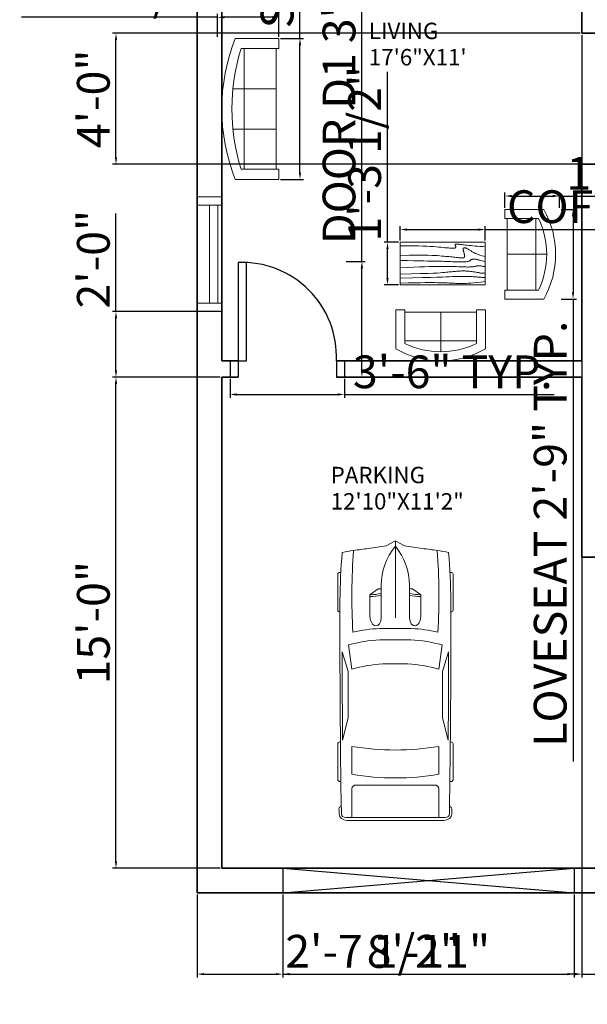
# Model space of a CAD drawing. Units: inches. Extents: x 2011 to 2548, y 530 to 1188.
# Tile 1 of 5: x 2011 to 2220, y 530 to 891. Entities that reach past the tile are written whole.
import ezdxf

# ---------------------------------------------------------------- set-up
doc = ezdxf.new("R2010")
doc.units = ezdxf.units.IN
for name, color, linetype, lineweight in [('A-ANNO-DIMS', 2, 'Continuous', 18), ('A-AREA-IDEN', 7, 'Continuous', 25), ('A-DOOR', 3, 'Continuous', 25), ('A-FURN', 8, 'Continuous', 18), ('A-GLAZ', 4, 'Continuous', 18), ('A-SITE-VEHC', 8, 'Continuous', 13), ('A-WALL', 7, 'Continuous', 35)]:
    doc.layers.add(name, color=color, linetype=linetype, lineweight=lineweight)
doc.styles.get("Standard").update_dxf_attribs({"font": 'arial.ttf'})
doc.dimstyles.new('ISO-25', dxfattribs={"dimtxt": 12, "dimasz": 2.5, "dimexe": 1.25, "dimexo": 0.625, "dimtad": 1, "dimdec": 1, "dimlunit": 3, "dimtxsty": 'Standard', "dimcen": 2.5, "dimadec": 0, "dimazin": 0, "dimtfac": 1, "dimtdec": 1, "dimtmove": 0, "dimatfit": 3, "dimfxl": 1, "dimarcsym": 0})

# ---------------------------------------------------------------- blocks, each defined once
blk = doc.blocks.new('Sofa - Roundback 7 ft.')
for p, q in [((-36.000027, -34), (-36.000027, -11.4696)), ((-12.00002, -32.4421), (-12.00003, -6.5971)), ((11.99997, -32.4421), (11.99998, -6.5971)), ((35.99998, -34), (35.99998, -11.4696)), ((-35.999844, -13.3819), (35.9998, -13.3819)), ((-36.000027, -32.4421), (35.99998, -32.4421))]:
    blk.add_line(p, q)
for points in [[(-36.000027, -34), (-42.000027, -34), (-42.000027, -8)], [(41.99998, -8), (41.99998, -34), (35.99998, -34)]]:
    blk.add_lwpolyline(points)
for centre, radius, start, end in [((0, -114.25), 114.25, 68.43141, 111.5686), ((-0.00001, -127.1968), 121.1968, 72.72033, 107.2797)]:
    blk.add_arc(centre, radius, start, end)
blk = doc.blocks.new('Table - Rectangular Woodgrain 60 x 30 in.')
for p, q in [((0, 0), (0, -30)), ((60, 0), (0, 0)), ((60, -30), (60, 0)), ((0, -30), (60, -30))]:
    blk.add_line(p, q)
for points in [[(0, -2.4), (4.8155, -2.418), (9.0302, -2.4688), (12.709, -2.5477), (15.9167, -2.65), (18.7181, -2.7711), (21.1781, -2.9063), (23.3616, -3.0508), (25.3333, -3.2), (27.1477, -3.3495), (28.8172, -3.4958), (30.3437, -3.636), (31.7291, -3.7667), (32.9756, -3.8849), (34.0849, -3.9875), (35.059, -4.0714), (35.9, -4.1334), (36.6114, -4.1711), (37.2041, -4.1854), (37.6906, -4.1779), (38.0833, -4.15), (38.3948, -4.1034), (38.6375, -4.0396), (38.8239, -3.9602), (38.9666, -3.8667), (39.0764, -3.7608), (39.1573, -3.6448), (39.2116, -3.521), (39.2416, -3.3917), (39.2498, -3.2593), (39.2385, -3.1261), (39.21, -2.9944), (39.1666, -2.8667), (39.111, -2.7447), (39.0468, -2.6281), (38.978, -2.5163), (38.9083, -2.4083), (38.8418, -2.3035), (38.7823, -2.201), (38.7337, -2.1001), (38.7, -2), (38.6844, -1.9003), (38.6875, -1.8021), (38.7094, -1.707), (38.75, -1.6167), (38.8094, -1.5326), (38.8875, -1.4563), (38.9844, -1.3893), (39.1, -1.3333), (39.2351, -1.2896), (39.3937, -1.2583), (39.5804, -1.2396), (39.8, -1.2333), (40.057, -1.2396), (40.3562, -1.2583), (40.7023, -1.2896), (41.1, -1.3333), (41.5547, -1.3895), (42.0755, -1.4573), (42.6721, -1.5361), (43.3542, -1.625), (44.1316, -1.7233), (45.014, -1.8302), (46.0114, -1.9449), (47.1333, -2.0667), (48.3862, -2.1947), (49.7625, -2.3281), (51.2513, -2.4663), (52.8416, -2.6083), (54.5226, -2.7535), (56.2833, -2.9011), (58.1127, -3.0501), (60, -3.2)], [(0, -9.2), (6.5759, -9.0858), (11.9385, -9.0365), (16.2527, -9.0418), (19.6833, -9.0917), (22.3952, -9.1759), (24.5531, -9.2844), (26.322, -9.4069), (27.8666, -9.5333), (29.3241, -9.6553), (30.7203, -9.7719), (32.0532, -9.8837), (33.3208, -9.9917), (34.5213, -10.0965), (35.6526, -10.199), (36.7128, -10.2999), (37.7, -10.4), (38.6129, -10.4996), (39.4531, -10.5969), (40.223, -10.6895), (40.925, -10.775), (41.5613, -10.8512), (42.1344, -10.9156), (42.6465, -10.966), (43.1, -11), (43.4976, -11.0158), (43.8437, -11.0136), (44.143, -10.9942), (44.4, -10.9583), (44.6195, -10.9069), (44.8062, -10.8406), (44.9648, -10.7603), (45.1, -10.6667), (45.2155, -10.5598), (45.3114, -10.4365), (45.3871, -10.2929), (45.4416, -10.125), (45.4743, -9.929), (45.4844, -9.7011), (45.4709, -9.4371), (45.4333, -9.1333), (45.3716, -8.7883), (45.2896, -8.4104), (45.1919, -8.0107), (45.0833, -7.6), (44.9685, -7.1893), (44.8521, -6.7896), (44.7388, -6.4117), (44.6333, -6.0667), (44.54, -5.7628), (44.4614, -5.4979), (44.4001, -5.2675), (44.3583, -5.0667), (44.3384, -4.8909), (44.3427, -4.7354), (44.3736, -4.5956), (44.4333, -4.4667), (44.5236, -4.3453), (44.6427, -4.2333), (44.7884, -4.1339), (44.9583, -4.05), (45.1501, -3.9849), (45.3614, -3.9417), (45.59, -3.9234), (45.8333, -3.9333), (46.0915, -3.9749), (46.3734, -4.0531), (46.6906, -4.1736), (47.0542, -4.3417), (47.4756, -4.5629), (47.9661, -4.8427), (48.5372, -5.1866), (49.2, -5.6), (49.9676, -6.0844), (50.8594, -6.625), (51.8965, -7.2031), (53.1, -7.8), (54.491, -8.3969), (56.0906, -8.975), (57.9199, -9.5156), (60, -10)], [(0, -12.8), (5.1847, -12.9322), (9.6213, -13.0323), (13.3963, -13.1059), (16.5958, -13.1583), (19.3063, -13.1952), (21.614, -13.2219), (23.6054, -13.2439), (25.3666, -13.2667), (26.9728, -13.2947), (28.4531, -13.3281), (29.8256, -13.3663), (31.1083, -13.4083), (32.3191, -13.4535), (33.476, -13.501), (34.597, -13.5501), (35.7, -13.6), (36.7984, -13.6497), (37.8875, -13.6979), (38.9578, -13.743), (40, -13.7833), (41.0047, -13.8174), (41.9625, -13.8438), (42.864, -13.8607), (43.7, -13.8667), (44.4631, -13.8604), (45.1552, -13.8417), (45.7801, -13.8104), (46.3416, -13.7667), (46.8439, -13.7104), (47.2906, -13.6417), (47.6858, -13.5604), (48.0333, -13.4667), (48.3375, -13.3608), (48.6042, -13.2448), (48.8396, -13.121), (49.05, -12.9917), (49.2417, -12.8593), (49.4208, -12.7261), (49.5937, -12.5944), (49.7667, -12.4667), (49.9452, -12.3451), (50.1323, -12.2313), (50.3303, -12.1268), (50.5416, -12.0333), (50.7686, -11.9524), (51.0135, -11.8854), (51.2788, -11.8341), (51.5666, -11.8), (51.8785, -11.7843), (52.2116, -11.7865), (52.562, -11.8059), (52.926, -11.8417), (53.2998, -11.8931), (53.6795, -11.9594), (54.0614, -12.0397), (54.4416, -12.1333), (54.8223, -12.2401), (55.2293, -12.3625), (55.6942, -12.5037), (56.2489, -12.6667), (56.9251, -12.8547), (57.7545, -13.0708), (58.7689, -13.3182), (60, -13.6)], [(0, -18), (5.124, -17.7273), (9.6609, -17.5057), (13.6705, -17.3303), (17.2125, -17.1958), (20.3467, -17.0973), (23.1328, -17.0297), (25.6307, -16.9878), (27.9, -16.9667), (29.9928, -16.9617), (31.9302, -16.9703), (33.7254, -16.9907), (35.3917, -17.0208), (36.9423, -17.0588), (38.3906, -17.1026), (39.7499, -17.1503), (41.0333, -17.2), (42.2519, -17.2496), (43.4073, -17.2969), (44.4986, -17.3395), (45.525, -17.375), (46.4858, -17.4012), (47.3802, -17.4156), (48.2074, -17.416), (48.9667, -17.4), (49.6583, -17.3662), (50.2872, -17.3167), (50.8595, -17.2547), (51.3812, -17.1833), (51.8584, -17.1057), (52.2971, -17.025), (52.7034, -16.9443), (53.0833, -16.8667), (53.443, -16.7951), (53.789, -16.7313), (54.128, -16.6768), (54.4666, -16.6334), (54.8115, -16.6024), (55.1693, -16.5854), (55.5465, -16.5841), (55.95, -16.6), (56.3828, -16.6337), (56.8346, -16.6823), (57.2915, -16.7418), (57.7396, -16.8084), (58.165, -16.878), (58.5539, -16.9469), (58.8924, -17.0111), (59.1666, -17.0667), (59.3679, -17.1107), (59.5078, -17.1438), (59.6032, -17.1675), (59.6708, -17.1833), (59.7275, -17.193), (59.7901, -17.1979), (59.8753, -17.1998), (60, -17.2)], [(0, -22.4), (8.0098, -22.2501), (14.4094, -22.1011), (19.4168, -21.9535), (23.25, -21.8083), (26.1269, -21.6663), (28.2656, -21.5281), (29.884, -21.3947), (31.2, -21.2667), (32.3967, -21.1448), (33.5172, -21.0292), (34.5697, -20.9198), (35.5625, -20.8167), (36.5037, -20.7198), (37.4015, -20.6292), (38.2642, -20.5448), (39.1, -20.4667), (39.9164, -20.3951), (40.7187, -20.3313), (41.5117, -20.2768), (42.3, -20.2333), (43.0883, -20.2024), (43.8812, -20.1854), (44.6836, -20.1841), (45.5, -20.2), (46.3328, -20.234), (47.1747, -20.2844), (48.0163, -20.3488), (48.8479, -20.425), (49.66, -20.5106), (50.4429, -20.6031), (51.1872, -20.7004), (51.8833, -20.8), (52.5246, -20.8999), (53.1166, -20.9995), (53.6681, -21.0983), (54.1875, -21.1958), (54.6834, -21.2919), (55.1646, -21.3859), (55.6394, -21.4777), (56.1167, -21.5667), (56.6028, -21.6515), (57.0961, -21.7266), (57.5929, -21.7852), (58.0896, -21.8208), (58.5823, -21.8268), (59.0674, -21.7964), (59.5412, -21.723), (60, -21.6)], [(0, -25.2), (8.6355, -25.0504), (15.7026, -24.9031), (21.4049, -24.7606), (25.9458, -24.625), (29.529, -24.4988), (32.3578, -24.3844), (34.6359, -24.284), (36.5667, -24.2), (38.3213, -24.1341), (39.9417, -24.0854), (41.437, -24.0523), (42.8167, -24.0333), (44.0901, -24.0268), (45.2667, -24.0313), (46.3557, -24.0451), (47.3667, -24.0667), (48.309, -24.0947), (49.1928, -24.1287), (50.0284, -24.168), (50.826, -24.2125), (51.5959, -24.2617), (52.3483, -24.3151), (53.0935, -24.3725), (53.8417, -24.4334), (54.6009, -24.497), (55.3699, -24.561), (56.1454, -24.6226), (56.9239, -24.6792), (57.7021, -24.7279), (58.4764, -24.7662), (59.2435, -24.7911), (60, -24.8)], [(0, -28.8), (5.6867, -28.6681), (10.45, -28.5698), (14.407, -28.5012), (17.675, -28.4584), (20.3711, -28.4374), (22.6125, -28.4344), (24.5164, -28.4455), (26.2, -28.4667), (27.762, -28.4947), (29.2276, -28.5281), (30.6033, -28.5663), (31.8958, -28.6084), (33.1118, -28.6535), (34.2578, -28.7011), (35.3405, -28.7501), (36.3666, -28.8), (37.3443, -28.8497), (38.288, -28.8974), (39.2137, -28.9412), (40.1375, -28.9792), (41.0753, -29.0093), (42.0432, -29.0297), (43.0572, -29.0384), (44.1333, -29.0333), (45.2936, -29.0114), (46.5843, -28.9641), (48.0579, -28.8816), (49.7666, -28.7542), (51.7629, -28.5721), (54.0989, -28.3255), (56.8272, -28.0048), (60, -27.6)]]:
    blk.add_lwpolyline(points)
blk = doc.blocks.new('Sofa - Roundback Loveseat 5 ft.')
for p, q in [((0, -32.44198), (0, -5.99998)), ((-24, -33.99998), (-24, -11.46958)), ((24.00004, -33.99998), (24.00004, -11.46958)), ((-23.9998, -13.38178), (23.99986, -13.38178)), ((-24, -32.44198), (24.00004, -32.44198))]:
    blk.add_line(p, q)
for points in [[(-24, -33.99998), (-30, -33.99998), (-30, -7.99998)], [(30.00004, -7.99998), (30.00004, -33.99998), (24.00004, -33.99998)]]:
    blk.add_lwpolyline(points)
for centre, radius, start, end in [((0, -60.24998), 60.24998, 60.13715, 119.8628), ((0, -61.38438), 55.38444, 64.32083, 115.6792)]:
    blk.add_arc(centre, radius, start, end)
blk = doc.blocks.new('*U11')
for p, q in [((21.1, 37.41), (21.1, 36.83)), ((46.55, 38.89), (22.35, 38.89)), ((47.8, 37.39), (47.8, 37.41)), ((87.99, 31.87), (74.76, 35.92)), ((134.31, 35.6), (119.29, 31.78)), ((135.45, 37.07), (135.45, 37.41)), ((136.7, 38.89), (160.9, 38.89)), ((162.15, 37.41), (162.15, 36.77)), ((186.47, -33.5), (186.47, 33.5)), ((70.03, 31.54), (86.41, 29.35)), ((138.42, 29.35), (157.25, 29.35)), ((186.47, 29.35), (167.01, 29.35)), ((188.4, -32.76), (188.4, 32.76)), ((164.52, 26.39), (164.52, -26.39)), ((32.27, 11.63), (36.13, 17.17)), ((36.13, 17.17), (50.94, 17.17)), ((29.77, 9.51), (51.68, 9.51)), ((32.12, 9.51), (32.12, 11.15)), ((58.92, -10.77), (58.92, 10.77)), ((66.55, -10.53), (66.55, 10.53)), ((82.74, 8.5), (82.74, -8.5)), ((186.47, -10.53), (186.47, 10.53)), ((3.27, 6.13), (0.1, 0.41)), ((0, 0), (51.68, 0)), ((0.1, -0.41), (3.27, -6.13)), ((29.77, -9.51), (51.68, -9.51)), ((32.12, -9.51), (32.12, -11.15)), ((32.27, -11.63), (36.13, -17.17)), ((36.13, -17.17), (50.94, -17.17)), ((86.41, -29.35), (70.03, -31.54)), ((87.99, -31.87), (74.76, -35.92)), ((134.31, -35.6), (119.29, -31.78)), ((157.25, -29.35), (138.42, -29.35)), ((167.01, -29.35), (186.47, -29.35)), ((21.1, -37.41), (21.1, -36.83)), ((46.55, -38.89), (22.35, -38.89)), ((47.8, -37.39), (47.8, -37.41)), ((135.45, -37.07), (135.45, -37.41)), ((136.7, -38.89), (160.9, -38.89)), ((162.15, -37.41), (162.15, -36.77))]:
    blk.add_line(p, q)
for centre, major_axis, ratio, start_param, end_param in [((266.03, -27.52), (0, 313.31), 0.842304, 1.367076, 1.39176), ((41.19, -490.86), (0, 528.23), 0.842304, 0.00281, 0.075598), ((22.35, 37.41), (0, -1.48), 0.842304, 3.141593, 4.712389), ((64.48, -10555.62), (0, 10593.03), 0.842304, -0.013397, 0.002797), ((46.55, 37.41), (0, 1.48), 0.842304, -1.570796, 0), ((64.48, -10555.62), (0, -10591.55), 0.842304, 3.133765, 3.140441), ((136.7, 37.41), (0, -1.48), 0.842304, 3.141593, 4.712389), ((160.9, 37.41), (0, 1.48), 0.842304, -1.570796, 0), ((180.63, 35.84), (0, 2.22), 0.842304, -0.013017, 1.249894), ((64.48, -10556.36), (0, 10595.31), 0.842304, -0.013397, -0.013017), ((183.98, 33.5), (0, -2.96), 0.842304, 1.570796, 3.128196), ((183.98, 32.76), (0, -5.25), 0.842304, 1.570796, 3.128196), ((259.18, -27.52), (0, -305.3), 0.842304, 4.528606, 4.561838), ((37.47, -593.96), (0, -623.33), 0.842304, 3.096046, 3.200911), ((134.4, 5.39), (0, -89.78), 0.842304, 4.449482, 4.652344), ((135.29, 5.39), (0, 81.77), 0.842304, 1.245306, 1.50788), ((149.6, 2.8), (0, -79.58), 0.842304, 4.372215, 4.640744), ((95.79, -3666.35), (0, -3698.24), 0.842304, 3.134049, 3.144098), ((17.08, 0), (0, 147.02), 0.842304, 4.511394, 4.913384), ((35.91, 0), (0, 147.02), 0.842304, 4.511394, 4.913384), ((167.01, 26.39), (0, 2.96), 0.842304, 0, 1.570796), ((-204.49, 52.4), (0, -250.96), 0.842304, 1.385369, 1.434372), ((13.04, 17.01), (0, 27.42), 0.842304, 4.435146, 4.718221), ((14.2, 17.01), (0, 27.42), 0.842304, 4.435146, 4.718221), ((50.79, 13.34), (6.34, -0.36), 0.603834, -1.395552, 1.581315), ((29.77, -46.66), (0, 56.17), 0.842304, 0, 0.590319), ((32.75, 11.15), (0, 0.74), 0.842304, 0.879714, 1.570796), ((0.62, 0), (0, -0.74), 0.842304, 4.131459, 5.293319), ((-204.49, -52.4), (0, 250.96), 0.842304, -1.434372, -1.385369), ((29.77, 46.66), (0, 56.17), 0.842304, 2.551274, 3.141593), ((32.75, -11.15), (0, -0.74), 0.842304, 4.712389, 5.403472), ((13.04, -17.01), (0, -27.42), 0.842304, 1.564964, 1.848039), ((14.2, -17.01), (0, -27.42), 0.842304, 1.564964, 1.848039), ((134.4, -5.39), (0, -89.78), 0.842304, -1.510751, -1.307889), ((135.29, -5.39), (0, -81.77), 0.842304, -1.50788, -1.245306), ((149.6, -2.8), (0, -79.58), 0.842304, -1.499151, -1.230623), ((259.18, 27.52), (0, 305.3), 0.842304, 1.721348, 1.754579), ((167.01, -26.39), (0, -2.96), 0.842304, 4.712389, 6.283185), ((266.03, 27.52), (0, 313.31), 0.842304, 1.749832, 1.774517), ((37.47, 593.96), (0, -623.33), 0.842304, -0.059319, 0.045547), ((95.79, 3666.35), (0, -3698.24), 0.842304, -0.002505, 0.007544), ((183.98, -32.76), (0, -5.25), 0.842304, 0.013397, 1.570796), ((41.19, 490.86), (0, -528.23), 0.842304, -0.075598, -0.00281), ((22.35, -37.41), (0, 1.48), 0.842304, 1.570796, 3.141593), ((64.48, 10555.62), (0, 10593.03), 0.842304, 3.138796, 3.15499), ((46.55, -37.41), (0, -1.48), 0.842304, 0, 1.570796), ((64.48, 10555.62), (0, -10591.55), 0.842304, 0.001152, 0.007828), ((136.7, -37.41), (0, -1.48), 0.842304, -1.570796, 0), ((160.9, -37.41), (0, 1.48), 0.842304, 3.141593, 4.712389), ((180.63, -35.84), (0, -2.22), 0.842304, -1.249894, 0.013017), ((64.48, 10556.36), (0, 10595.31), 0.842304, 3.15461, 3.15499), ((183.98, -33.5), (0, 2.96), 0.842304, 3.15499, 4.712389)]:
    blk.add_ellipse(centre, major_axis=major_axis, ratio=ratio, start_param=start_param, end_param=end_param)
at = {"extrusion": (0, 0, -1)}
blk.add_ellipse((50.79, -13.34), major_axis=(6.34, 0.36), ratio=0.603834, start_param=-1.395552, end_param=1.581315, dxfattribs=at)
blk = doc.blocks.new('WIN-36IN')
for p, q in [((0, 42), (9, 42)), ((0, 3), (0, 39)), ((0, 39), (9, 39)), ((1.5, 39), (1.5, 3)), ((4.5, 39), (4.5, 3)), ((9, 39), (9, 3)), ((9, 3), (0, 3)), ((9, 0), (0, 0))]:
    blk.add_line(p, q)
blk = doc.blocks.new('DOOR-SWING-36IN-6IN-JAMB')
for p, q in [((0, 6), (0, 0)), ((3, 6), (3, 0)), ((39, 6), (39, 0)), ((42, 6), (42, 0))]:
    blk.add_line(p, q)
blk.add_lwpolyline([(3, 6), (6, 6), (6, 42), (3, 42)], close=True)
blk.add_arc((4.5, 7.5), 34.53, 357.5104, 92.4896)
blk = doc.blocks.new('*D21')
at = {"layer": 'A-ANNO-DIMS', "color": 0, "lineweight": -2, "transparency": 16777216}
for p, q in [((2136.89, 802.78), (2136.89, 988.08)), ((2131.15, 802.78), (2138.14, 802.78)), ((2136.89, 762.86), (2136.89, 800.28)), ((2131.15, 760.36), (2138.14, 760.36))]:
    blk.add_line(p, q, dxfattribs=at)
at = {"layer": 'A-ANNO-DIMS', "color": 0, "transparency": 16777216}
for points in [[(2136.47, 800.28), (2137.31, 800.28), (2136.89, 802.78)], [(2136.47, 762.86), (2137.31, 762.86), (2136.89, 760.36)]]:
    blk.add_solid(points, dxfattribs=at)
at = {"layer": 'Defpoints', "color": 0, "transparency": 16777216}
for p in [(2130.53, 802.78), (2136.89, 802.78), (2130.53, 760.36)]:
    blk.add_point(p, dxfattribs=at)
at = {"layer": 'A-ANNO-DIMS', "color": 0, "transparency": 16777216, "insert": (2130.05, 896.68), "char_height": 12, "attachment_point": 5, "rotation": 90}
blk.add_mtext('DOOR D1 3\'-6 1/2" TYP.', dxfattribs=at)
blk = doc.blocks.new('*D22')
at = {"layer": 'A-ANNO-DIMS', "color": 0, "lineweight": -2, "transparency": 16777216}
for p, q in [((2088.53, 759.73), (2088.53, 752.75)), ((2130.53, 759.73), (2130.53, 752.75)), ((2091.03, 754), (2128.03, 754)), ((2130.53, 754), (2207.41, 754))]:
    blk.add_line(p, q, dxfattribs=at)
at = {"layer": 'A-ANNO-DIMS', "color": 0, "transparency": 16777216}
for points in [[(2091.03, 754.41), (2091.03, 753.58), (2088.53, 754)], [(2128.03, 754.41), (2128.03, 753.58), (2130.53, 754)]]:
    blk.add_solid(points, dxfattribs=at)
at = {"layer": 'Defpoints', "color": 0, "transparency": 16777216}
for p in [(2088.53, 760.36), (2130.53, 760.36), (2130.53, 754)]:
    blk.add_point(p, dxfattribs=at)
at = {"layer": 'A-ANNO-DIMS', "color": 0, "transparency": 16777216, "insert": (2170.22, 760.75), "char_height": 12, "attachment_point": 5}
blk.add_mtext('3\'-6" TYP.', dxfattribs=at)
blk = doc.blocks.new('*D27')
at = {"layer": 'A-ANNO-DIMS', "color": 0, "lineweight": -2, "transparency": 16777216}
for p, q in [((2210, 821.8), (2215.55, 821.8)), ((2214.3, 819.3), (2214.3, 791.47)), ((2210, 788.97), (2215.55, 788.97)), ((2214.3, 788.97), (2214.3, 619.44))]:
    blk.add_line(p, q, dxfattribs=at)
at = {"layer": 'A-ANNO-DIMS', "color": 0, "transparency": 16777216}
for points in [[(2213.88, 819.3), (2214.72, 819.3), (2214.3, 821.8)], [(2213.88, 791.47), (2214.72, 791.47), (2214.3, 788.97)]]:
    blk.add_solid(points, dxfattribs=at)
at = {"layer": 'Defpoints', "color": 0, "transparency": 16777216}
for p in [(2209.38, 821.8), (2209.38, 788.97), (2214.3, 788.97)]:
    blk.add_point(p, dxfattribs=at)
at = {"layer": 'A-ANNO-DIMS', "color": 0, "transparency": 16777216, "insert": (2207.47, 702.96), "char_height": 12, "attachment_point": 5, "rotation": 90}
blk.add_mtext('LOVESEAT 2\'-9" TYP.', dxfattribs=at)
blk = doc.blocks.new('*D28')
at = {"layer": 'A-ANNO-DIMS', "color": 0, "lineweight": -2, "transparency": 16777216}
for p, q in [((2189.31, 822.43), (2189.31, 827.98)), ((2191.81, 826.73), (2206.88, 826.73)), ((2209.38, 822.43), (2209.38, 827.98)), ((2209.38, 826.73), (2285.14, 826.73))]:
    blk.add_line(p, q, dxfattribs=at)
at = {"layer": 'A-ANNO-DIMS', "color": 0, "transparency": 16777216}
for points in [[(2191.81, 827.15), (2191.81, 826.31), (2189.31, 826.73)], [(2206.88, 827.15), (2206.88, 826.31), (2209.38, 826.73)]]:
    blk.add_solid(points, dxfattribs=at)
at = {"layer": 'Defpoints', "color": 0, "transparency": 16777216}
for p in [(2209.38, 826.73), (2189.31, 821.8), (2209.38, 821.8)]:
    blk.add_point(p, dxfattribs=at)
at = {"layer": 'A-ANNO-DIMS', "color": 0, "transparency": 16777216, "insert": (2248.51, 833.48), "char_height": 12, "attachment_point": 5}
blk.add_mtext('1\'-8" TYP.', dxfattribs=at)
blk = doc.blocks.new('*D37')
at = {"layer": 'A-ANNO-DIMS', "color": 0, "lineweight": -2, "transparency": 16777216}
for p, q in [((2114.19, 884.5), (2114.19, 998.36)), ((2107.06, 884.5), (2115.44, 884.5)), ((2114.19, 835.34), (2114.19, 882)), ((2107.06, 832.84), (2115.44, 832.84))]:
    blk.add_line(p, q, dxfattribs=at)
at = {"layer": 'A-ANNO-DIMS', "color": 0, "transparency": 16777216}
for points in [[(2113.77, 882), (2114.61, 882), (2114.19, 884.5)], [(2113.77, 835.34), (2114.61, 835.34), (2114.19, 832.84)]]:
    blk.add_solid(points, dxfattribs=at)
at = {"layer": 'Defpoints', "color": 0, "transparency": 16777216}
for p in [(2106.44, 884.5), (2114.19, 884.5), (2106.44, 832.84)]:
    blk.add_point(p, dxfattribs=at)
at = {"layer": 'A-ANNO-DIMS', "color": 0, "transparency": 16777216, "insert": (2107.35, 942.68), "char_height": 12, "attachment_point": 5, "rotation": 90}
blk.add_mtext('SOFA 4\'-3 1/2"', dxfattribs=at)
blk = doc.blocks.new('*D38')
at = {"layer": 'A-ANNO-DIMS', "color": 0, "lineweight": -2, "transparency": 16777216}
for p, q in [((2083.89, 892.25), (2012.08, 892.25)), ((2083.89, 885.13), (2083.89, 893.5)), ((2103.94, 892.25), (2086.39, 892.25)), ((2106.44, 885.13), (2106.44, 893.5))]:
    blk.add_line(p, q, dxfattribs=at)
at = {"layer": 'A-ANNO-DIMS', "color": 0, "transparency": 16777216}
for points in [[(2086.39, 892.67), (2086.39, 891.84), (2083.89, 892.25)], [(2103.94, 892.67), (2103.94, 891.84), (2106.44, 892.25)]]:
    blk.add_solid(points, dxfattribs=at)
at = {"layer": 'Defpoints', "color": 0, "transparency": 16777216}
for p in [(2083.89, 892.25), (2083.89, 884.5), (2106.44, 884.5)]:
    blk.add_point(p, dxfattribs=at)
at = {"layer": 'A-ANNO-DIMS', "color": 0, "transparency": 16777216, "insert": (2046.73, 899.08), "char_height": 12, "attachment_point": 5}
blk.add_mtext('1\'-10 1/2"', dxfattribs=at)
blk = doc.blocks.new('*D39')
at = {"layer": 'A-ANNO-DIMS', "color": 0, "lineweight": -2, "transparency": 16777216}
for p, q in [((2150.94, 810.39), (2150.94, 815.69)), ((2182.11, 810.39), (2182.11, 815.69)), ((2153.44, 814.44), (2179.61, 814.44)), ((2182.11, 814.44), (2348.03, 814.44))]:
    blk.add_line(p, q, dxfattribs=at)
at = {"layer": 'A-ANNO-DIMS', "color": 0, "transparency": 16777216}
for points in [[(2153.44, 814.85), (2153.44, 814.02), (2150.94, 814.44)], [(2179.61, 814.85), (2179.61, 814.02), (2182.11, 814.44)]]:
    blk.add_solid(points, dxfattribs=at)
at = {"layer": 'Defpoints', "color": 0, "transparency": 16777216}
for p in [(2182.11, 814.44), (2150.94, 809.76), (2182.11, 809.76)]:
    blk.add_point(p, dxfattribs=at)
at = {"layer": 'A-ANNO-DIMS', "color": 0, "transparency": 16777216, "insert": (2266.32, 821.27), "char_height": 12, "attachment_point": 5}
blk.add_mtext('COFFEE TABLE 2\'-7"', dxfattribs=at)
blk = doc.blocks.new('*D40')
at = {"layer": 'A-ANNO-DIMS', "color": 0, "lineweight": -2, "transparency": 16777216}
for p, q in [((2146.26, 809.76), (2146.26, 872.24)), ((2150.31, 809.76), (2145.01, 809.76)), ((2146.26, 796.68), (2146.26, 807.26)), ((2150.31, 794.18), (2145.01, 794.18))]:
    blk.add_line(p, q, dxfattribs=at)
at = {"layer": 'A-ANNO-DIMS', "color": 0, "transparency": 16777216}
for points in [[(2145.85, 807.26), (2146.68, 807.26), (2146.26, 809.76)], [(2145.85, 796.68), (2146.68, 796.68), (2146.26, 794.18)]]:
    blk.add_solid(points, dxfattribs=at)
at = {"layer": 'Defpoints', "color": 0, "transparency": 16777216}
for p in [(2146.26, 809.76), (2150.94, 809.76), (2150.94, 794.18)]:
    blk.add_point(p, dxfattribs=at)
at = {"layer": 'A-ANNO-DIMS', "color": 0, "transparency": 16777216, "insert": (2139.43, 842.25), "char_height": 12, "attachment_point": 5, "rotation": 90}
blk.add_mtext('1\'-3 1/2"', dxfattribs=at)
blk = doc.blocks.new('*D41')
at = {"layer": 'A-ANNO-DIMS', "color": 0, "lineweight": -2, "transparency": 16777216}
for p, q in [((2076.53, 570.73), (2076.53, 540.31)), ((2107.85, 570.73), (2107.85, 540.31)), ((2079.03, 541.56), (2105.35, 541.56)), ((2107.85, 541.56), (2171.66, 541.56))]:
    blk.add_line(p, q, dxfattribs=at)
at = {"layer": 'A-ANNO-DIMS', "color": 0, "transparency": 16777216}
for points in [[(2079.03, 541.98), (2079.03, 541.14), (2076.53, 541.56)], [(2105.35, 541.98), (2105.35, 541.14), (2107.85, 541.56)]]:
    blk.add_solid(points, dxfattribs=at)
at = {"layer": 'Defpoints', "color": 0, "transparency": 16777216}
for p in [(2076.53, 571.36), (2107.85, 571.36), (2107.85, 541.56)]:
    blk.add_point(p, dxfattribs=at)
at = {"layer": 'A-ANNO-DIMS', "color": 0, "transparency": 16777216, "insert": (2141, 548.39), "char_height": 12, "attachment_point": 5}
blk.add_mtext('2\'-7 1/2"', dxfattribs=at)
blk = doc.blocks.new('*D42')
at = {"layer": 'A-ANNO-DIMS', "color": 0, "lineweight": -2, "transparency": 16777216}
for p, q in [((2107.85, 570.73), (2107.85, 540.31)), ((2214.72, 570.73), (2214.72, 540.31)), ((2110.35, 541.56), (2212.22, 541.56))]:
    blk.add_line(p, q, dxfattribs=at)
at = {"layer": 'A-ANNO-DIMS', "color": 0, "transparency": 16777216}
for points in [[(2110.35, 541.98), (2110.35, 541.14), (2107.85, 541.56)], [(2212.22, 541.98), (2212.22, 541.14), (2214.72, 541.56)]]:
    blk.add_solid(points, dxfattribs=at)
at = {"layer": 'Defpoints', "color": 0, "transparency": 16777216}
for p in [(2107.85, 571.36), (2214.72, 571.36), (2214.72, 541.56)]:
    blk.add_point(p, dxfattribs=at)
at = {"layer": 'A-ANNO-DIMS', "color": 0, "transparency": 16777216, "insert": (2161.28, 548.31), "char_height": 12, "attachment_point": 5}
blk.add_mtext('8\'-11"', dxfattribs=at)
blk = doc.blocks.new('*D45')
at = {"layer": 'A-ANNO-DIMS', "color": 0, "lineweight": -2, "transparency": 16777216}
for p, q in [((2084.9, 760.36), (2045.48, 760.36)), ((2046.73, 582.86), (2046.73, 757.86)), ((2084.9, 580.36), (2045.48, 580.36))]:
    blk.add_line(p, q, dxfattribs=at)
at = {"layer": 'A-ANNO-DIMS', "color": 0, "transparency": 16777216}
for points in [[(2046.31, 757.86), (2047.14, 757.86), (2046.73, 760.36)], [(2046.31, 582.86), (2047.14, 582.86), (2046.73, 580.36)]]:
    blk.add_solid(points, dxfattribs=at)
at = {"layer": 'Defpoints', "color": 0, "transparency": 16777216}
for p in [(2046.73, 760.36), (2085.53, 760.36), (2085.53, 580.36)]:
    blk.add_point(p, dxfattribs=at)
at = {"layer": 'A-ANNO-DIMS', "color": 0, "transparency": 16777216, "insert": (2039.98, 670.36), "char_height": 12, "attachment_point": 5, "rotation": 90}
blk.add_mtext('15\'-0"', dxfattribs=at)
blk = doc.blocks.new('*D53')
at = {"layer": 'A-ANNO-DIMS', "color": 0, "lineweight": -2, "transparency": 16777216}
for p, q in [((2046.73, 784.41), (2046.73, 820.27)), ((2084.9, 784.41), (2045.48, 784.41)), ((2046.73, 762.86), (2046.73, 781.91)), ((2084.9, 760.36), (2045.48, 760.36))]:
    blk.add_line(p, q, dxfattribs=at)
at = {"layer": 'A-ANNO-DIMS', "color": 0, "transparency": 16777216}
for points in [[(2046.31, 781.91), (2047.14, 781.91), (2046.73, 784.41)], [(2046.31, 762.86), (2047.14, 762.86), (2046.73, 760.36)]]:
    blk.add_solid(points, dxfattribs=at)
at = {"layer": 'Defpoints', "color": 0, "transparency": 16777216}
for p in [(2046.73, 784.41), (2085.53, 784.41), (2085.53, 760.36)]:
    blk.add_point(p, dxfattribs=at)
at = {"layer": 'A-ANNO-DIMS', "color": 0, "transparency": 16777216, "insert": (2039.98, 803.59), "char_height": 12, "attachment_point": 5, "rotation": 90}
blk.add_mtext('2\'-0"', dxfattribs=at)
blk = doc.blocks.new('*D54')
at = {"layer": 'A-ANNO-DIMS', "color": 0, "lineweight": -2, "transparency": 16777216}
for p, q in [((2223.53, 891.73), (2223.53, 540.31)), ((2217.53, 885.73), (2217.53, 540.31)), ((2215.03, 541.56), (2212.53, 541.56)), ((2217.53, 541.56), (2223.53, 541.56)), ((2226.03, 541.56), (2261.68, 541.56))]:
    blk.add_line(p, q, dxfattribs=at)
at = {"layer": 'A-ANNO-DIMS', "color": 0, "transparency": 16777216}
for points in [[(2215.03, 541.98), (2215.03, 541.14), (2217.53, 541.56)], [(2226.03, 541.98), (2226.03, 541.14), (2223.53, 541.56)]]:
    blk.add_solid(points, dxfattribs=at)
at = {"layer": 'Defpoints', "color": 0, "transparency": 16777216}
for p in [(2223.53, 892.36), (2217.53, 886.36), (2223.53, 541.56)]:
    blk.add_point(p, dxfattribs=at)
at = {"layer": 'A-ANNO-DIMS', "color": 0, "transparency": 16777216, "insert": (2245.1, 548.31), "char_height": 12, "attachment_point": 5}
blk.add_mtext('0\'-6"', dxfattribs=at)
blk = doc.blocks.new('*D57')
at = {"layer": 'A-ANNO-DIMS', "color": 0, "lineweight": -2, "transparency": 16777216}
for p, q in [((2216.9, 886.36), (2045.48, 886.36)), ((2046.73, 840.86), (2046.73, 883.86)), ((2216.9, 838.36), (2045.48, 838.36))]:
    blk.add_line(p, q, dxfattribs=at)
at = {"layer": 'A-ANNO-DIMS', "color": 0, "transparency": 16777216}
for points in [[(2046.31, 883.86), (2047.14, 883.86), (2046.73, 886.36)], [(2046.31, 840.86), (2047.14, 840.86), (2046.73, 838.36)]]:
    blk.add_solid(points, dxfattribs=at)
at = {"layer": 'Defpoints', "color": 0, "transparency": 16777216}
for p in [(2046.73, 886.36), (2217.53, 886.36), (2217.53, 838.36)]:
    blk.add_point(p, dxfattribs=at)
at = {"layer": 'A-ANNO-DIMS', "color": 0, "transparency": 16777216, "insert": (2039.98, 862.36), "char_height": 12, "attachment_point": 5, "rotation": 90}
blk.add_mtext('4\'-0"', dxfattribs=at)

msp = doc.modelspace()

# ---------------------------------------------------------------- linework, layer by layer
at = {"layer": 'A-DOOR'}
for p, q in [((2107.85, 580.36), (2107.85, 571.36)), ((2107.85, 580.36), (2214.72, 571.36)), ((2107.85, 571.36), (2214.72, 580.36)), ((2214.72, 580.36), (2214.72, 571.36))]:
    msp.add_line(p, q, dxfattribs=at)
at = {"layer": 'A-WALL'}
for p, q in [((2085.53, 976.36), (2085.53, 766.36)), ((2217.53, 976.36), (2217.53, 886.36)), ((2229.53, 886.36), (2217.53, 886.36)), ((2217.53, 838.36), (2217.53, 766.36)), ((2229.53, 838.36), (2217.53, 838.36)), ((2091.53, 766.36), (2085.53, 766.36)), ((2217.53, 766.36), (2127.53, 766.36)), ((2085.53, 760.36), (2085.53, 580.36)), ((2091.53, 760.36), (2085.53, 760.36)), ((2217.53, 760.36), (2127.53, 760.36)), ((2217.53, 760.36), (2217.53, 694.36)), ((2367.53, 694.36), (2217.53, 694.36)), ((2085.53, 580.36), (2367.53, 580.36))]:
    msp.add_line(p, q, dxfattribs=at)
msp.add_lwpolyline([(2076.53, 1060.36), (2076.53, 571.36), (2376.53, 571.36), (2376.53, 1111.36), (2076.53, 1111.36), (2076.53, 1096.36)], dxfattribs=at)

# ---------------------------------------------------------------- block references
at = {"layer": 'A-DOOR'}
msp.add_blockref('DOOR-SWING-36IN-6IN-JAMB', (2088.53, 760.36), dxfattribs=at)
at = {"layer": 'A-FURN'}
for name, p, xscale, yscale, zscale, rotation in [('Sofa - Roundback 7 ft.', (2085.53, 858.67), 0.6150722271576684, 0.6150722271576684, 0.6150722271576684, 90), ('Sofa - Roundback Loveseat 5 ft.', (2207.92, 805.39), 0.5471718440280605, 0.5471718440280605, 0.5471718440280605, 270), ('Sofa - Roundback Loveseat 5 ft.', (2165.79, 766.36), 0.5471718440280605, 0.5471718440280605, 0.5471718440280605, 180)]:
    msp.add_blockref(name, p, dxfattribs=dict(at, xscale=xscale, yscale=yscale, zscale=zscale, rotation=rotation))
at = {"layer": 'A-FURN', "xscale": 0.5194406169888572, "yscale": 0.5194406169888572, "zscale": 0.5194406169888572}
msp.add_blockref('Table - Rectangular Woodgrain 60 x 30 in.', (2150.94, 809.76), dxfattribs=at)
at = {"layer": 'A-GLAZ', "rotation": 180}
msp.add_blockref('WIN-36IN', (2085.53, 826.41), dxfattribs=at)
at = {"layer": 'A-SITE-VEHC', "xscale": 0.5433754347557287, "yscale": 0.5433754347557287, "zscale": 0.5433754347557287, "rotation": 270}
msp.add_blockref('*U11', (2149.16, 700.25), dxfattribs=at)

# ---------------------------------------------------------------- texts
at = {"layer": 'A-AREA-IDEN'}
for s, p in [('LIVING', (2139.43, 884.25)), ('17\'6"X11\'', (2139.43, 874.61)), ('PARKING', (2125.43, 721.48)), ('12\'10"X11\'2"', (2125.43, 711.84))]:
    msp.add_text(s, height=6, dxfattribs=at).set_placement(p)

# ---------------------------------------------------------------- dimensions: what is measured, and where the dimension line sits
at = {"layer": 'A-ANNO-DIMS'}
for base, p1, p2, angle, text, picture, middle in [((2114.19, 884.5), (2106.44, 832.84), (2106.44, 884.5), 90, 'SOFA <>', '*D37', (2107.35, 942.68)), ((2136.89, 802.78), (2130.53, 760.36), (2130.53, 802.78), 90, 'DOOR D1 <> TYP.', '*D21', (2130.05, 896.68)), ((2214.3, 788.97), (2209.38, 821.8), (2209.38, 788.97), 270, 'LOVESEAT <> TYP.', '*D27', (2207.47, 702.96))]:
    dim = msp.add_linear_dim(base=base, p1=p1, p2=p2, angle=angle, text=text, dimstyle='ISO-25', override={"dimdec": 1, "dimlfac": 1, "dimrnd": 0, "dimzin": 1, "dimdsep": 46, "dimlunit": 4, "dimfrac": 2}, dxfattribs=at)
    dim.commit()
    dim.dimension.update_dxf_attribs({"geometry": picture, "text_midpoint": middle})
for base, p1, p2, angle, picture, middle in [((2083.8868, 892.2546), (2106.4394, 884.5047), (2083.8868, 884.5047), 180, '*D38', (2046.7345, 899.0843)), ((2046.73, 886.36), (2217.53, 838.36), (2217.53, 886.36), 90, '*D57', (2039.98, 862.36)), ((2146.26, 809.76), (2150.94, 794.18), (2150.94, 809.76), 90, '*D40', (2139.43, 842.25)), ((2046.727, 784.4133), (2085.527, 760.3587), (2085.527, 784.4133), 90, '*D53', (2039.9751, 803.5902)), ((2046.73, 760.36), (2085.53, 580.36), (2085.53, 760.36), 90, '*D45', (2039.98, 670.36))]:
    dim = msp.add_linear_dim(base=base, p1=p1, p2=p2, angle=angle, dimstyle='ISO-25', override={"dimdec": 1, "dimlfac": 1, "dimrnd": 0, "dimzin": 1, "dimdsep": 46, "dimlunit": 4, "dimfrac": 2}, dxfattribs=at)
    dim.commit()
    dim.dimension.update_dxf_attribs({"geometry": picture, "text_midpoint": middle})
for base, p1, p2, picture, middle in [((2223.53, 541.56), (2217.53, 886.36), (2223.53, 892.36), '*D54', (2245.1, 548.31)), ((2107.85, 541.56), (2076.53, 571.36), (2107.85, 571.36), '*D41', (2141, 548.39)), ((2214.72, 541.56), (2107.85, 571.36), (2214.72, 571.36), '*D42', (2161.28, 548.31))]:
    dim = msp.add_linear_dim(base=base, p1=p1, p2=p2, dimstyle='ISO-25', override={"dimdec": 1, "dimlfac": 1, "dimrnd": 0, "dimzin": 1, "dimdsep": 46, "dimlunit": 4, "dimfrac": 2}, dxfattribs=at)
    dim.commit()
    dim.dimension.update_dxf_attribs({"geometry": picture, "text_midpoint": middle})
for base, p1, p2, text, picture, middle in [((2182.11, 814.44), (2150.94, 809.76), (2182.11, 809.76), 'COFFEE TABLE <>', '*D39', (2266.32, 821.27)), ((2209.38, 826.73), (2189.31, 821.8), (2209.38, 821.8), '<> TYP.', '*D28', (2248.51, 833.48)), ((2130.53, 754), (2088.53, 760.36), (2130.53, 760.36), '<> TYP.', '*D22', (2170.22, 760.75))]:
    dim = msp.add_linear_dim(base=base, p1=p1, p2=p2, text=text, dimstyle='ISO-25', override={"dimdec": 1, "dimlfac": 1, "dimrnd": 0, "dimzin": 1, "dimdsep": 46, "dimlunit": 4, "dimfrac": 2}, dxfattribs=at)
    dim.commit()
    dim.dimension.update_dxf_attribs({"geometry": picture, "text_midpoint": middle})

doc.saveas('drawing.dxf')
